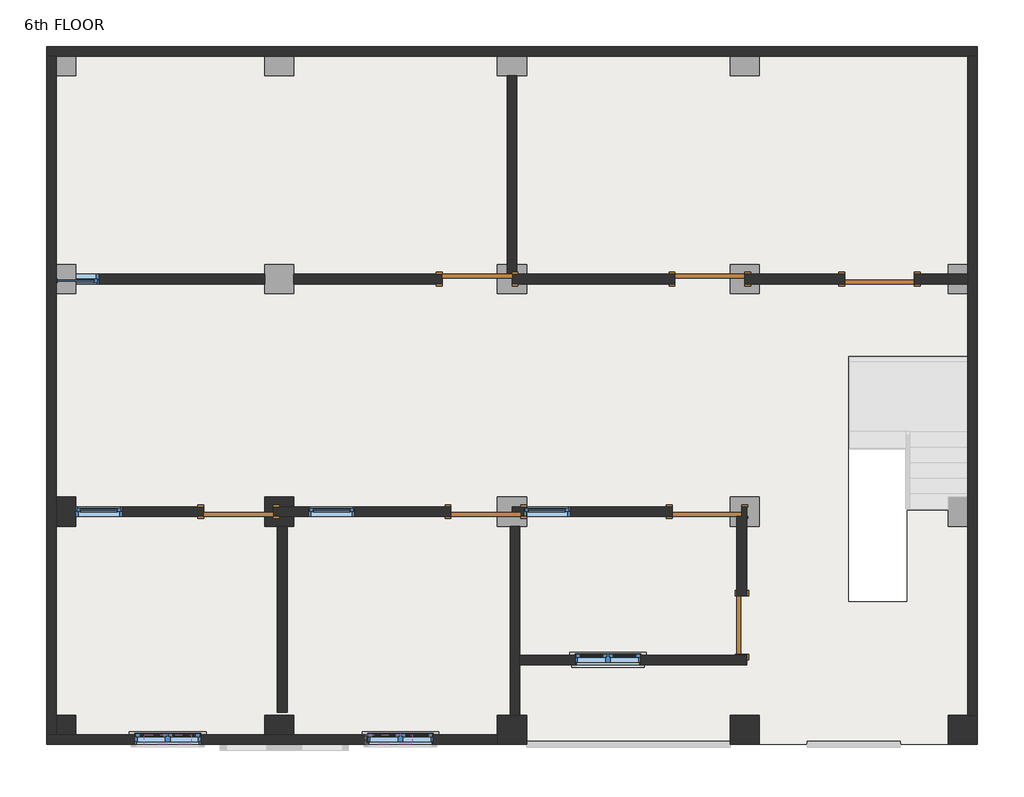
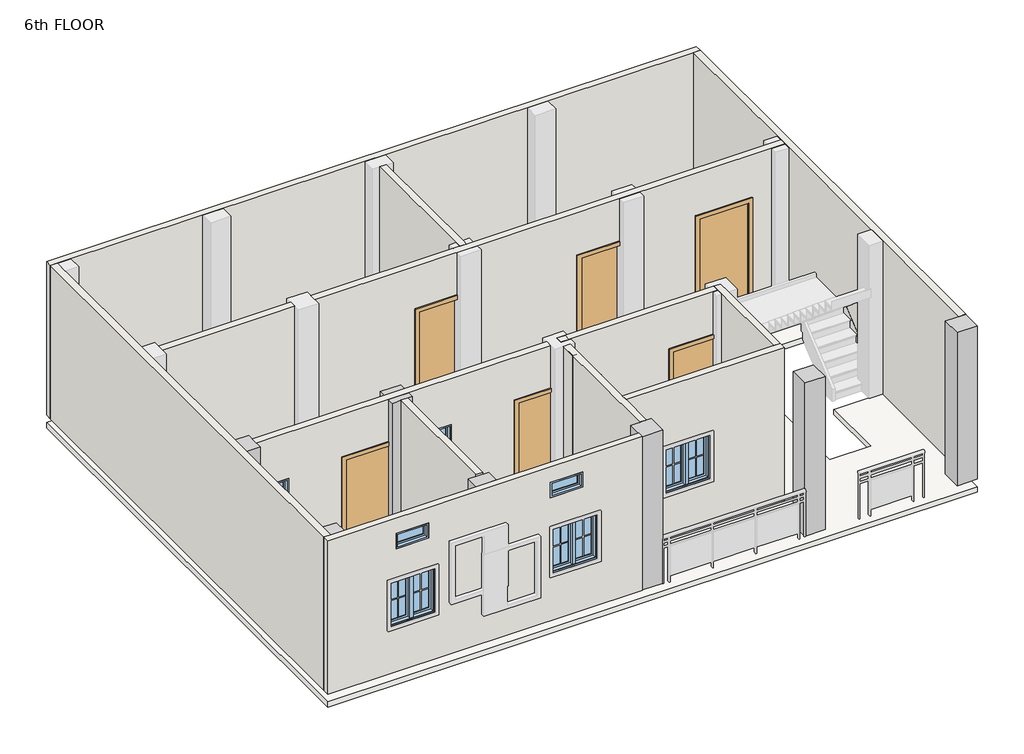
# One storey, part 1 of 2: 15 walls, 9 windows, 7 columns, 7 doors, 1 slab.
"""IFC4 building model written with IfcOpenShell, lengths in millimetres."""

from ifc_helpers import new_model, si_unit, frame, origin, place, context, project, spatial, polyline, outline, extrude, faceted_brep, transform, mapped, element, save
from components import door_e00f436c, door_a1797ceb, window_4c2727af, window_0bf3737e, window_78893e6c, window_0d9958e7

model = new_model("IFC4")

# Units and contexts
model_context = context("Model", 3, world=origin())
ifc_project = project(units=[si_unit("LENGTHUNIT", "METRE", prefix="MILLI")], contexts=[model_context])

# Site, building, storey
site = spatial("IfcSite", under=ifc_project)
building = spatial("IfcBuilding", under=site)
storey = spatial("IfcBuildingStorey", under=building, Name="6th FLOOR", Elevation=18135.6)

# Columns
placement = place(None, origin())
element("IfcColumn", 1, ObjectType="column family : column family", at=placement, inside=storey, context=model_context, shape_type="Brep", body=[
    faceted_brep([(-12576.097125, 2486.2065522, 18140.6), (-12957.097125, 2486.2065522, 18140.6), (-12957.097125, 2867.2065522, 18140.6), (-12576.097125, 2867.2065522, 18140.6), (-12576.097125, 2740.2065522, 18140.6), (-12842.797125, 2740.2065522, 18140.6), (-12842.797125, 2613.2065522, 18140.6), (-12576.097125, 2613.2065522, 18140.6), (-12576.097125, 2486.2065522, 21178.6), (-12576.097125, 2613.2065522, 21178.6), (-12957.097125, 2486.2065522, 21178.6), (-12957.097125, 2613.2065522, 21178.6), (-12957.097125, 2613.2065522, 20269.2), (-12957.097125, 2740.2065522, 20269.2), (-12957.097125, 2740.2065522, 21178.6), (-12957.097125, 2867.2065522, 21178.6), (-12576.097125, 2867.2065522, 21178.6), (-12842.797125, 2613.2065522, 20269.2), (-12842.797125, 2740.2065522, 20269.2), (-12576.097125, 2740.2065522, 21178.6)], [[[0, 1, 2, 3, 4, 5, 6, 7]], [[8, 0, 7, 9]], [[1, 0, 8, 10]], [[2, 1, 10, 11, 12, 13, 14, 15]], [[3, 2, 15, 16]], [[10, 8, 9, 11]], [[6, 17, 12, 11, 9, 7]], [[13, 18, 5, 4, 19, 14]], [[3, 16, 19, 4]], [[16, 15, 14, 19]], [[17, 18, 13, 12]], [[18, 17, 6, 5]]]),
])
element("IfcColumn", 2, ObjectType="column family : column family", at=placement, inside=storey, context=model_context, shape_type="SweptSolid", body=[
    extrude(outline(polyline([(-15433.597125, 2867.2065522), (-15433.597125, 2486.2065522), (-15687.597125, 2486.2065522), (-15687.597125, 2867.2065522), (-15433.597125, 2867.2065522)])), frame((0.0, 0.0, 18140.6), z_axis=(0.0, 0.0, 1.0), x_axis=(1.0, 0.0, 0.0)), (0.0, 0.0, 1.0), 3038.0),
])
element("IfcColumn", 3, ObjectType="column family : column family", at=placement, inside=storey, context=model_context, shape_type="SweptSolid", body=[
    extrude(outline(polyline([(-15433.597125, 9.7065522), (-15433.597125, -244.2934478), (-15687.597125, -244.2934478), (-15687.597125, 9.7065522), (-15433.597125, 9.7065522)])), frame((0.0, 0.0, 18140.6), z_axis=(0.0, 0.0, 1.0), x_axis=(1.0, 0.0, 0.0)), (0.0, 0.0, 1.0), 3038.0),
])
element("IfcColumn", 4, ObjectType="column family : column family", at=placement, inside=storey, context=model_context, shape_type="SweptSolid", body=[
    extrude(outline(polyline([(-3622.597125, 9.7065522), (-3622.597125, -371.2934478), (-4003.597125, -371.2934478), (-4003.597125, 9.7065522), (-3622.597125, 9.7065522)])), frame((0.0, 0.0, 18140.6), z_axis=(0.0, 0.0, 1.0), x_axis=(1.0, 0.0, 0.0)), (0.0, 0.0, 1.0), 3038.0),
])
element("IfcColumn", 5, ObjectType="column family : column family", at=placement, inside=storey, context=model_context, shape_type="SweptSolid", body=[
    extrude(outline(polyline([(-6480.097125, 9.7065522), (-6480.097125, -371.2934478), (-6861.097125, -371.2934478), (-6861.097125, 9.7065522), (-6480.097125, 9.7065522)])), frame((0.0, 0.0, 18140.6), z_axis=(0.0, 0.0, 1.0), x_axis=(1.0, 0.0, 0.0)), (0.0, 0.0, 1.0), 3038.0),
])
element("IfcColumn", 6, ObjectType="column family : column family", at=placement, inside=storey, context=model_context, shape_type="SweptSolid", body=[
    extrude(outline(polyline([(-9528.097125, 9.7065522), (-9528.097125, -371.2934478), (-9909.097125, -371.2934478), (-9909.097125, 9.7065522), (-9528.097125, 9.7065522)])), frame((0.0, 0.0, 18140.6), z_axis=(0.0, 0.0, 1.0), x_axis=(1.0, 0.0, 0.0)), (0.0, 0.0, 1.0), 3038.0),
])
element("IfcColumn", 7, ObjectType="column family : column family", at=placement, inside=storey, context=model_context, shape_type="SweptSolid", body=[
    extrude(outline(polyline([(-12957.097125, 9.7065522), (-12576.097125, 9.7065522), (-12576.097125, -244.2934478), (-12957.097125, -244.2934478), (-12957.097125, 9.7065522)])), frame((0.0, 0.0, 18140.6), z_axis=(0.0, 0.0, 1.0), x_axis=(1.0, 0.0, 0.0)), (0.0, 0.0, 1.0), 3038.0),
])

# Doors
door_shape = door_e00f436c(model_context)
element("IfcDoor", 8, ObjectType="Single-Flush : 30\" x 80\"", at=placement, inside=storey, context=model_context, shape_type="MappedRepresentation", body=[
    mapped(door_shape, transform((-6708.697125, 1190.8065522, 18135.6), x_axis=(0.0, -1.0, 0.0), y_axis=(1.0, 0.0, 0.0), z_axis=(0.0, 0.0, 1.0))),
])
door_2_shape = door_a1797ceb(model_context)
element("IfcDoor", 9, ObjectType="Single-Flush : 36\" x 84\"", at=placement, inside=storey, context=model_context, shape_type="MappedRepresentation", body=[
    mapped(door_2_shape, transform((-10175.797125, 5724.7065522, 18135.6), x_axis=(1.0, 0.0, 0.0), y_axis=(0.0, 1.0, 0.0), z_axis=(0.0, 0.0, 1.0))),
])
element("IfcDoor", 10, ObjectType="Single-Flush : 36\" x 84\"", at=placement, inside=storey, context=model_context, shape_type="MappedRepresentation", body=[
    mapped(door_2_shape, transform((-10061.497125, 2676.7065522, 18135.6), x_axis=(-1.0, 0.0, 0.0), y_axis=(0.0, -1.0, 0.0), z_axis=(0.0, 0.0, 1.0))),
])
element("IfcDoor", 11, ObjectType="Single-Flush : 36\" x 84\"", at=placement, inside=storey, context=model_context, shape_type="MappedRepresentation", body=[
    mapped(door_2_shape, transform((-13299.997125, 2676.7065522, 18135.6), x_axis=(-1.0, 0.0, 0.0), y_axis=(0.0, -1.0, 0.0), z_axis=(0.0, 0.0, 1.0))),
])
element("IfcDoor", 12, ObjectType="Single-Flush : 36\" x 84\"", at=placement, inside=storey, context=model_context, shape_type="MappedRepresentation", body=[
    mapped(door_2_shape, transform((-7127.797125, 5724.7065522, 18135.6), x_axis=(1.0, 0.0, 0.0), y_axis=(0.0, 1.0, 0.0), z_axis=(0.0, 0.0, 1.0))),
])
element("IfcDoor", 13, ObjectType="Single-Flush : 36\" x 84\"", at=placement, inside=storey, context=model_context, shape_type="MappedRepresentation", body=[
    mapped(door_2_shape, transform((-7165.897125, 2676.7065522, 18135.6), x_axis=(-1.0, 0.0, 0.0), y_axis=(0.0, -1.0, 0.0), z_axis=(0.0, 0.0, 1.0))),
])
element("IfcDoor", 14, ObjectType="Single-Flush : 36\" x 84\"", at=placement, inside=storey, context=model_context, shape_type="MappedRepresentation", body=[
    mapped(door_2_shape, transform((-4905.297125, 5724.7065522, 18135.6), x_axis=(-1.0, 0.0, 0.0), y_axis=(0.0, -1.0, 0.0), z_axis=(0.0, 0.0, 1.0))),
])

# Slab
element("IfcSlab", 15, ObjectType="Generic - 4\"", at=placement, inside=storey, context=model_context, shape_type="SweptSolid", body=[
    extrude(outline(polyline([(-3622.597125, 8772.7065522), (-3622.597125, -371.2934478), (-15814.597125, -371.2934478), (-15814.597125, 8772.7065522), (-3622.597125, 8772.7065522)]), holes=[polyline([(-3734.357125, 4711.0719226), (-5310.2646464, 4711.0719226), (-5310.2646464, 1502.3126957), (-4547.7736682, 1502.3126957), (-4547.7736682, 2699.911213), (-3734.357125, 2699.911213), (-3734.357125, 4711.0719226)])]), frame((0.0, 0.0, 17881.6), z_axis=(0.0, 0.0, 1.0), x_axis=(1.0, 0.0, 0.0)), (0.0, 0.0, 1.0), 101.6),
])

# Walls
element("IfcWall", 16, ObjectType="Generic - 5\"", at=placement, inside=storey, context=model_context, shape_type="Brep", body=[
    faceted_brep([(-15814.597125, 8645.7065522, 18135.6), (-15687.597125, 8645.7065522, 18135.6), (-3749.597125, 8645.7065522, 18135.6), (-3622.597125, 8645.7065522, 18135.6), (-3622.597125, 8645.7065522, 21183.6), (-3749.597125, 8645.7065522, 21183.6), (-15687.597125, 8645.7065522, 21183.6), (-15814.597125, 8645.7065522, 21183.6), (-15814.597125, 8772.7065522, 18135.6), (-15814.597125, 8772.7065522, 21183.6), (-3622.597125, 8772.7065522, 21183.6), (-3622.597125, 8772.7065522, 18135.6)], [[[0, 1, 2, 3, 4, 5, 6, 7]], [[8, 9, 10, 11]], [[3, 2, 1, 0, 8, 11]], [[7, 6, 5, 4, 10, 9]], [[4, 3, 11, 10]], [[0, 7, 9, 8]]]),
])
element("IfcWall", 17, ObjectType="Generic - 5\"", at=placement, inside=storey, context=model_context, shape_type="Brep", body=[
    faceted_brep([(-3749.597125, 8645.7065522, 18135.6), (-3749.597125, 5788.2065522, 18135.6), (-3749.597125, 5661.2065522, 18135.6), (-3749.597125, 9.7065522, 18135.6), (-3749.597125, 9.7065522, 21183.6), (-3749.597125, 5661.2065522, 21183.6), (-3749.597125, 5788.2065522, 21183.6), (-3749.597125, 8645.7065522, 21183.6), (-3622.597125, 8645.7065522, 18135.6), (-3622.597125, 8645.7065522, 21183.6), (-3622.597125, 9.7065522, 21183.6), (-3622.597125, 9.7065522, 21178.6), (-3622.597125, 9.7065522, 18140.6), (-3622.597125, 9.7065522, 18135.6)], [[[0, 1, 2, 3, 4, 5, 6, 7]], [[8, 9, 10, 11, 12, 13]], [[3, 2, 1, 0, 8, 13]], [[4, 3, 13, 12, 11, 10]], [[7, 6, 5, 4, 10, 9]], [[0, 7, 9, 8]]]),
])
element("IfcWall", 18, ObjectType="Generic - 5\"", at=placement, inside=storey, context=model_context, shape_type="Brep", body=[
    faceted_brep([(-9909.097125, -244.2934478, 18135.6), (-15687.597125, -244.2934478, 18135.6), (-15814.597125, -244.2934478, 18135.6), (-15814.597125, -244.2934478, 21183.6), (-15687.597125, -244.2934478, 21183.6), (-9909.097125, -244.2934478, 21183.6), (-13795.297125, -244.2934478, 19964.4), (-14658.897125, -244.2934478, 19964.4), (-14658.897125, -244.2934478, 19050.0), (-13795.297125, -244.2934478, 19050.0), (-10747.297125, -244.2934478, 19964.4), (-11610.897125, -244.2934478, 19964.4), (-11610.897125, -244.2934478, 19050.0), (-10747.297125, -244.2934478, 19050.0), (-13922.297125, -244.2934478, 20878.8), (-14531.897125, -244.2934478, 20878.8), (-14531.897125, -244.2934478, 20574.0), (-13922.297125, -244.2934478, 20574.0), (-11026.697125, -244.2934478, 20878.8), (-11636.297125, -244.2934478, 20878.8), (-11636.297125, -244.2934478, 20574.0), (-11026.697125, -244.2934478, 20574.0), (-9909.097125, -371.2934478, 18135.6), (-9909.097125, -371.2934478, 18140.6), (-9909.097125, -371.2934478, 21178.6), (-9909.097125, -371.2934478, 21183.6), (-15814.597125, -371.2934478, 21183.6), (-15814.597125, -371.2934478, 18135.6), (-13795.297125, -371.2934478, 19964.4), (-13795.297125, -371.2934478, 19050.0), (-14658.897125, -371.2934478, 19050.0), (-14658.897125, -371.2934478, 19964.4), (-10747.297125, -371.2934478, 19964.4), (-10747.297125, -371.2934478, 19050.0), (-11610.897125, -371.2934478, 19050.0), (-11610.897125, -371.2934478, 19964.4), (-13922.297125, -371.2934478, 20878.8), (-13922.297125, -371.2934478, 20574.0), (-14531.897125, -371.2934478, 20574.0), (-14531.897125, -371.2934478, 20878.8), (-11026.697125, -371.2934478, 20878.8), (-11026.697125, -371.2934478, 20574.0), (-11636.297125, -371.2934478, 20574.0), (-11636.297125, -371.2934478, 20878.8)], [[[0, 1, 2, 3, 4, 5], [6, 7, 8, 9], [10, 11, 12, 13], [14, 15, 16, 17], [18, 19, 20, 21]], [[22, 23, 24, 25, 26, 27], [28, 29, 30, 31], [32, 33, 34, 35], [36, 37, 38, 39], [40, 41, 42, 43]], [[2, 1, 0, 22, 27]], [[5, 4, 3, 26, 25]], [[0, 5, 25, 24, 23, 22]], [[3, 2, 27, 26]], [[29, 28, 6, 9]], [[30, 29, 9, 8]], [[31, 30, 8, 7]], [[28, 31, 7, 6]], [[33, 32, 10, 13]], [[34, 33, 13, 12]], [[35, 34, 12, 11]], [[32, 35, 11, 10]], [[37, 36, 14, 17]], [[38, 37, 17, 16]], [[39, 38, 16, 15]], [[36, 39, 15, 14]], [[41, 40, 18, 21]], [[42, 41, 21, 20]], [[43, 42, 20, 19]], [[40, 43, 19, 18]]]),
])
element("IfcWall", 19, ObjectType="Generic - 5\"", at=placement, inside=storey, context=model_context, shape_type="Brep", body=[
    faceted_brep([(-15687.597125, -244.2934478, 18135.6), (-15687.597125, 8645.7065522, 18135.6), (-15687.597125, 8645.7065522, 18140.6), (-15687.597125, 8645.7065522, 21178.6), (-15687.597125, 8645.7065522, 21183.6), (-15687.597125, -244.2934478, 21183.6), (-15687.597125, -244.2934478, 21178.6), (-15687.597125, -244.2934478, 18140.6), (-15814.597125, -244.2934478, 18135.6), (-15814.597125, -244.2934478, 21183.6), (-15814.597125, 8645.7065522, 21183.6), (-15814.597125, 8645.7065522, 18135.6)], [[[0, 1, 2, 3, 4, 5, 6, 7]], [[8, 9, 10, 11]], [[1, 0, 8, 11]], [[5, 4, 10, 9]], [[4, 3, 2, 1, 11, 10]], [[0, 7, 6, 5, 9, 8]]]),
])
element("IfcWall", 20, ObjectType="Generic - 5\"", at=placement, inside=storey, context=model_context, shape_type="SweptSolid", body=[
    extrude(outline(polyline([(18135.6, -15433.597125), (18135.6, -12957.097125), (21183.6, -12957.097125), (21183.6, -15433.597125), (20269.2, -15433.597125), (20269.2, -15128.797125), (18440.4, -15128.797125), (18440.4, -15433.597125), (18135.6, -15433.597125)])), frame((0.0, 5661.2065522, 0.0), z_axis=(0.0, 1.0, 0.0), x_axis=(0.0, 0.0, 1.0)), (0.0, 0.0, 1.0), 127.0),
])
element("IfcWall", 21, ObjectType="Generic - 5\"", at=placement, inside=storey, context=model_context, shape_type="Brep", body=[
    faceted_brep([(-9782.097125, 8391.7065522, 18135.6), (-9782.097125, 5788.2065522, 18135.6), (-9782.097125, 5788.2065522, 18140.6), (-9782.097125, 5788.2065522, 20269.2), (-9782.097125, 5788.2065522, 21178.6), (-9782.097125, 5788.2065522, 21183.6), (-9782.097125, 8391.7065522, 21183.6), (-9655.097125, 8391.7065522, 18135.6), (-9655.097125, 8391.7065522, 21183.6), (-9655.097125, 5788.2065522, 21183.6), (-9655.097125, 5788.2065522, 21178.6), (-9655.097125, 5788.2065522, 18140.6), (-9655.097125, 5788.2065522, 18135.6), (-9718.597125, 5788.2065522, 18135.6)], [[[0, 1, 2, 3, 4, 5, 6]], [[7, 8, 9, 10, 11, 12]], [[1, 0, 7, 12, 13]], [[6, 5, 9, 8]], [[0, 6, 8, 7]], [[5, 4, 3, 2, 1, 13, 12, 11, 10, 9]]]),
])
element("IfcWall", 22, ObjectType="Generic - 5\"", at=placement, inside=storey, context=model_context, shape_type="Brep", body=[
    faceted_brep([(-6670.597125, 5661.2065522, 18135.6), (-5362.497125, 5661.2065522, 18135.6), (-5362.497125, 5661.2065522, 20269.2), (-4448.097125, 5661.2065522, 20269.2), (-4448.097125, 5661.2065522, 18135.6), (-3749.597125, 5661.2065522, 18135.6), (-3749.597125, 5661.2065522, 18140.6), (-3749.597125, 5661.2065522, 21178.6), (-3749.597125, 5661.2065522, 21183.6), (-12576.097125, 5661.2065522, 21183.6), (-12576.097125, 5661.2065522, 18135.6), (-10632.997125, 5661.2065522, 18135.6), (-10632.997125, 5661.2065522, 20269.2), (-9909.097125, 5661.2065522, 20269.2), (-9718.597125, 5661.2065522, 20269.2), (-9718.597125, 5661.2065522, 18140.6), (-9718.597125, 5661.2065522, 18135.6), (-7584.997125, 5661.2065522, 18135.6), (-7584.997125, 5661.2065522, 20269.2), (-6861.097125, 5661.2065522, 20269.2), (-6670.597125, 5661.2065522, 20269.2), (-6670.597125, 5661.2065522, 18140.6), (-5362.497125, 5788.2065522, 20269.2), (-5362.497125, 5788.2065522, 18135.6), (-6670.597125, 5788.2065522, 18135.6), (-6670.597125, 5788.2065522, 18140.6), (-6670.597125, 5788.2065522, 20269.2), (-6861.097125, 5788.2065522, 20269.2), (-7584.997125, 5788.2065522, 20269.2), (-7584.997125, 5788.2065522, 18135.6), (-9655.097125, 5788.2065522, 18135.6), (-9718.597125, 5788.2065522, 18135.6), (-9718.597125, 5788.2065522, 18140.6), (-9718.597125, 5788.2065522, 20269.2), (-9782.097125, 5788.2065522, 20269.2), (-9909.097125, 5788.2065522, 20269.2), (-10632.997125, 5788.2065522, 20269.2), (-10632.997125, 5788.2065522, 18135.6), (-12576.097125, 5788.2065522, 18135.6), (-12576.097125, 5788.2065522, 21183.6), (-9782.097125, 5788.2065522, 21183.6), (-9655.097125, 5788.2065522, 21183.6), (-3749.597125, 5788.2065522, 21183.6), (-3749.597125, 5788.2065522, 21178.6), (-3749.597125, 5788.2065522, 18140.6), (-3749.597125, 5788.2065522, 18135.6), (-4448.097125, 5788.2065522, 18135.6), (-4448.097125, 5788.2065522, 20269.2)], [[[0, 1, 2, 3, 4, 5, 6, 7, 8, 9, 10, 11, 12, 13, 14, 15, 16, 17, 18, 19, 20, 21]], [[22, 23, 24, 25, 26, 27, 28, 29, 30, 31, 32, 33, 34, 35, 36, 37, 38, 39, 40, 41, 42, 43, 44, 45, 46, 47]], [[11, 10, 38, 37]], [[17, 16, 31, 30, 29]], [[46, 45, 5, 4]], [[24, 23, 1, 0]], [[9, 8, 42, 41, 40, 39]], [[10, 9, 39, 38]], [[8, 7, 6, 5, 45, 44, 43, 42]], [[33, 32, 31, 16, 15, 14]], [[36, 35, 34, 33, 14, 13, 12]], [[37, 36, 12, 11]], [[26, 25, 24, 0, 21, 20]], [[28, 27, 26, 20, 19, 18]], [[29, 28, 18, 17]], [[2, 1, 23, 22]], [[3, 2, 22, 47]], [[4, 3, 47, 46]]]),
])
element("IfcWall", 23, ObjectType="Generic - 5\"", at=placement, inside=storey, context=model_context, shape_type="Brep", body=[
    faceted_brep([(-14823.997125, 2613.2065522, 18440.4), (-15433.597125, 2613.2065522, 18440.4), (-15433.597125, 2613.2065522, 18135.6), (-13757.197125, 2613.2065522, 18135.6), (-13757.197125, 2613.2065522, 20269.2), (-12957.097125, 2613.2065522, 20269.2), (-12842.797125, 2613.2065522, 20269.2), (-12842.797125, 2613.2065522, 18140.6), (-12842.797125, 2613.2065522, 18135.6), (-10518.697125, 2613.2065522, 18135.6), (-10518.697125, 2613.2065522, 20269.2), (-9909.097125, 2613.2065522, 20269.2), (-9909.097125, 2613.2065522, 21183.6), (-15433.597125, 2613.2065522, 21183.6), (-15433.597125, 2613.2065522, 20269.2), (-14823.997125, 2613.2065522, 20269.2), (-12385.597125, 2613.2065522, 20269.2), (-11775.997125, 2613.2065522, 20269.2), (-11775.997125, 2613.2065522, 18440.4), (-12385.597125, 2613.2065522, 18440.4), (-15433.597125, 2740.2065522, 18135.6), (-15433.597125, 2740.2065522, 18440.4), (-14823.997125, 2740.2065522, 18440.4), (-14823.997125, 2740.2065522, 20269.2), (-15433.597125, 2740.2065522, 20269.2), (-15433.597125, 2740.2065522, 21183.6), (-9909.097125, 2740.2065522, 21183.6), (-9909.097125, 2740.2065522, 20269.2), (-10518.697125, 2740.2065522, 20269.2), (-10518.697125, 2740.2065522, 18135.6), (-12842.797125, 2740.2065522, 18135.6), (-12842.797125, 2740.2065522, 18140.6), (-12842.797125, 2740.2065522, 20269.2), (-12957.097125, 2740.2065522, 20269.2), (-13757.197125, 2740.2065522, 20269.2), (-13757.197125, 2740.2065522, 18135.6), (-12385.597125, 2740.2065522, 20269.2), (-12385.597125, 2740.2065522, 18440.4), (-11775.997125, 2740.2065522, 18440.4), (-11775.997125, 2740.2065522, 20269.2)], [[[0, 1, 2, 3, 4, 5, 6, 7, 8, 9, 10, 11, 12, 13, 14, 15], [16, 17, 18, 19]], [[20, 21, 22, 23, 24, 25, 26, 27, 28, 29, 30, 31, 32, 33, 34, 35], [36, 37, 38, 39]], [[30, 29, 9, 8]], [[20, 35, 3, 2]], [[26, 12, 11, 27]], [[13, 12, 26, 25]], [[14, 13, 25, 24]], [[2, 1, 21, 20]], [[28, 10, 9, 29]], [[10, 28, 27, 11]], [[4, 3, 35, 34]], [[6, 5, 4, 34, 33, 32]], [[8, 7, 6, 32, 31, 30]], [[22, 21, 1, 0]], [[23, 22, 0, 15]], [[24, 23, 15, 14]], [[37, 36, 16, 19]], [[38, 37, 19, 18]], [[39, 38, 18, 17]], [[36, 39, 17, 16]]]),
])
element("IfcWall", 24, ObjectType="Generic - 5\"", at=placement, inside=storey, context=model_context, shape_type="Brep", body=[
    faceted_brep([(-9616.997125, 9.7065522, 18135.6), (-9616.997125, 670.1065522, 18135.6), (-9616.997125, 797.1065522, 18135.6), (-9616.997125, 2486.2065522, 18135.6), (-9616.997125, 2486.2065522, 21183.6), (-9616.997125, 797.1065522, 21183.6), (-9616.997125, 670.1065522, 21183.6), (-9616.997125, 9.7065522, 21183.6), (-9743.997125, 9.7065522, 18135.6), (-9743.997125, 9.7065522, 21183.6), (-9743.997125, 2486.2065522, 21183.6), (-9743.997125, 2486.2065522, 18135.6)], [[[0, 1, 2, 3, 4, 5, 6, 7]], [[8, 9, 10, 11]], [[3, 2, 1, 0, 8, 11]], [[4, 3, 11, 10]], [[7, 6, 5, 4, 10, 9]], [[0, 7, 9, 8]]]),
])
element("IfcWall", 25, ObjectType="Generic - 5\"", at=placement, inside=storey, context=model_context, shape_type="SweptSolid", body=[
    extrude(outline(polyline([(-9743.997125, 2181.4065522), (-9743.997125, 2486.2065522), (-9616.997125, 2486.2065522), (-9616.997125, 2181.4065522), (-9743.997125, 2181.4065522)])), frame((0.0, 0.0, 18135.6), z_axis=(0.0, 0.0, 1.0), x_axis=(1.0, 0.0, 0.0)), (0.0, 0.0, 1.0), 3048.0),
])
element("IfcWall", 26, ObjectType="Generic - 5\"", at=placement, inside=storey, context=model_context, shape_type="Brep", body=[
    faceted_brep([(-6772.197125, 2613.2065522, 21183.6), (-9718.597125, 2613.2065522, 21183.6), (-9718.597125, 2613.2065522, 21178.6), (-9718.597125, 2613.2065522, 18140.6), (-9718.597125, 2613.2065522, 18135.6), (-7623.097125, 2613.2065522, 18135.6), (-7623.097125, 2613.2065522, 20269.2), (-6861.097125, 2613.2065522, 20269.2), (-6772.197125, 2613.2065522, 20269.2), (-6772.197125, 2613.2065522, 21178.6), (-9566.197125, 2613.2065522, 20269.2), (-9528.097125, 2613.2065522, 20269.2), (-8956.597125, 2613.2065522, 20269.2), (-8956.597125, 2613.2065522, 18440.4), (-9528.097125, 2613.2065522, 18440.4), (-9566.197125, 2613.2065522, 18440.4), (-9718.597125, 2740.2065522, 21183.6), (-6772.197125, 2740.2065522, 21183.6), (-6772.197125, 2740.2065522, 20269.2), (-6861.097125, 2740.2065522, 20269.2), (-7623.097125, 2740.2065522, 20269.2), (-7623.097125, 2740.2065522, 18135.6), (-9718.597125, 2740.2065522, 18135.6), (-9718.597125, 2740.2065522, 18140.6), (-9718.597125, 2740.2065522, 21178.6), (-9566.197125, 2740.2065522, 20269.2), (-9566.197125, 2740.2065522, 18440.4), (-9528.097125, 2740.2065522, 18440.4), (-8956.597125, 2740.2065522, 18440.4), (-8956.597125, 2740.2065522, 20269.2), (-9528.097125, 2740.2065522, 20269.2)], [[[0, 1, 2, 3, 4, 5, 6, 7, 8, 9], [10, 11, 12, 13, 14, 15]], [[16, 17, 18, 19, 20, 21, 22, 23, 24], [25, 26, 27, 28, 29, 30]], [[4, 22, 21, 5]], [[1, 0, 17, 16]], [[4, 3, 2, 1, 16, 24, 23, 22]], [[26, 25, 10, 15]], [[28, 27, 26, 15, 14, 13]], [[29, 28, 13, 12]], [[25, 30, 29, 12, 11, 10]], [[20, 6, 5, 21]], [[6, 20, 19, 18, 8, 7]], [[17, 0, 9, 8, 18]]]),
])
element("IfcWall", 27, ObjectType="Generic - 5\"", at=placement, inside=storey, context=model_context, shape_type="Brep", body=[
    faceted_brep([(-6645.197125, 797.1065522, 18135.6), (-6645.197125, 809.8065522, 18135.6), (-6645.197125, 809.8065522, 20167.6), (-6645.197125, 1571.8065522, 20167.6), (-6645.197125, 1571.8065522, 18135.6), (-6645.197125, 2740.2065522, 18135.6), (-6645.197125, 2740.2065522, 18140.6), (-6645.197125, 2740.2065522, 21178.6), (-6645.197125, 2740.2065522, 21183.6), (-6645.197125, 797.1065522, 21183.6), (-6772.197125, 809.8065522, 20167.6), (-6772.197125, 809.8065522, 18135.6), (-6772.197125, 797.1065522, 18135.6), (-6772.197125, 797.1065522, 21183.6), (-6772.197125, 2613.2065522, 21183.6), (-6772.197125, 2740.2065522, 21183.6), (-6772.197125, 2740.2065522, 20269.2), (-6772.197125, 2613.2065522, 20269.2), (-6772.197125, 2613.2065522, 18140.6), (-6772.197125, 2613.2065522, 18135.6), (-6772.197125, 1571.8065522, 18135.6), (-6772.197125, 1571.8065522, 20167.6), (-6708.697125, 2613.2065522, 18135.6), (-6708.697125, 2740.2065522, 18135.6), (-6708.697125, 2613.2065522, 20269.2), (-6708.697125, 2613.2065522, 18140.6), (-6708.697125, 2740.2065522, 20269.2), (-6708.697125, 2740.2065522, 18140.6)], [[[0, 1, 2, 3, 4, 5, 6, 7, 8, 9]], [[10, 11, 12, 13, 14, 15, 16, 17, 18, 19, 20, 21]], [[20, 19, 22, 23, 5, 4]], [[12, 11, 1, 0]], [[9, 8, 15, 14, 13]], [[24, 25, 22, 19, 18, 17]], [[26, 24, 17, 16]], [[22, 25, 24, 26, 27, 23]], [[8, 7, 6, 5, 23, 27, 26, 16, 15]], [[0, 9, 13, 12]], [[2, 1, 11, 10]], [[3, 2, 10, 21]], [[4, 3, 21, 20]]]),
])
element("IfcWall", 28, ObjectType="Generic - 5\"", at=placement, inside=storey, context=model_context, shape_type="Brep", body=[
    faceted_brep([(-9718.597125, 2613.2065522, 18135.6), (-9566.197125, 2613.2065522, 18135.6), (-9566.197125, 2613.2065522, 18440.4), (-9566.197125, 2613.2065522, 20269.2), (-9566.197125, 2613.2065522, 21183.6), (-9718.597125, 2613.2065522, 21183.6), (-9718.597125, 2613.2065522, 21178.6), (-9718.597125, 2613.2065522, 18140.6), (-9718.597125, 2740.2065522, 18135.6), (-9718.597125, 2740.2065522, 18140.6), (-9718.597125, 2740.2065522, 21178.6), (-9718.597125, 2740.2065522, 21183.6), (-9566.197125, 2740.2065522, 21183.6), (-9566.197125, 2740.2065522, 20269.2), (-9566.197125, 2740.2065522, 18440.4), (-9566.197125, 2740.2065522, 18135.6)], [[[0, 1, 2, 3, 4, 5, 6, 7]], [[8, 9, 10, 11, 12, 13, 14, 15]], [[1, 0, 8, 15]], [[4, 3, 2, 1, 15, 14, 13, 12]], [[5, 4, 12, 11]], [[0, 7, 6, 5, 11, 10, 9, 8]]]),
])
element("IfcWall", 29, ObjectType="Generic - 5\"", at=placement, inside=storey, context=model_context, shape_type="SweptSolid", body=[
    extrude(outline(polyline([(-12791.997125, 47.8065522), (-12791.997125, 2486.2065522), (-12664.997125, 2486.2065522), (-12664.997125, 47.8065522), (-12791.997125, 47.8065522)])), frame((0.0, 0.0, 18135.6), z_axis=(0.0, 0.0, 1.0), x_axis=(1.0, 0.0, 0.0)), (0.0, 0.0, 1.0), 3048.0),
])
element("IfcWall", 30, ObjectType="Generic - 5\"", at=placement, inside=storey, context=model_context, shape_type="Brep", body=[
    faceted_brep([(-9616.997125, 670.1065522, 18135.6), (-6645.197125, 670.1065522, 18135.6), (-6645.197125, 670.1065522, 21183.6), (-9616.997125, 670.1065522, 21183.6), (-8029.497125, 670.1065522, 19964.4), (-8029.497125, 670.1065522, 19050.0), (-8893.097125, 670.1065522, 19050.0), (-8893.097125, 670.1065522, 19964.4), (-9616.997125, 797.1065522, 18135.6), (-9616.997125, 797.1065522, 21183.6), (-6772.197125, 797.1065522, 21183.6), (-6645.197125, 797.1065522, 21183.6), (-6645.197125, 797.1065522, 18135.6), (-6772.197125, 797.1065522, 18135.6), (-8029.497125, 797.1065522, 19964.4), (-8893.097125, 797.1065522, 19964.4), (-8893.097125, 797.1065522, 19050.0), (-8029.497125, 797.1065522, 19050.0)], [[[0, 1, 2, 3], [4, 5, 6, 7]], [[8, 9, 10, 11, 12, 13], [14, 15, 16, 17]], [[1, 0, 8, 13, 12]], [[3, 2, 11, 10, 9]], [[0, 3, 9, 8]], [[2, 1, 12, 11]], [[5, 4, 14, 17]], [[6, 5, 17, 16]], [[7, 6, 16, 15]], [[4, 7, 15, 14]]]),
])

# Windows
window_shape = window_4c2727af(model_context)
element("IfcWindow", 31, ObjectType="Fixed : 24\" x 12\"", at=placement, inside=storey, context=model_context, shape_type="MappedRepresentation", body=[
    mapped(window_shape, transform((-14188.997125, -307.7934478, 19659.6), x_axis=(1.0, 0.0, 0.0), y_axis=(0.0, 1.0, 0.0), z_axis=(0.0, 0.0, 1.0))),
])
element("IfcWindow", 32, ObjectType="Fixed : 24\" x 12\"", at=placement, inside=storey, context=model_context, shape_type="MappedRepresentation", body=[
    mapped(window_shape, transform((-11293.397125, -307.7934478, 19659.6), x_axis=(1.0, 0.0, 0.0), y_axis=(0.0, 1.0, 0.0), z_axis=(0.0, 0.0, 1.0))),
])
window_2_shape = window_0bf3737e(model_context)
element("IfcWindow", 33, ObjectType="Fixed : 24\" x 72\"", at=placement, inside=storey, context=model_context, shape_type="MappedRepresentation", body=[
    mapped(window_2_shape, transform((-15471.697125, 5724.7065522, 18135.6), x_axis=(-1.0, 0.0, 0.0), y_axis=(0.0, -1.0, 0.0), z_axis=(0.0, 0.0, 1.0))),
])
window_3_shape = window_78893e6c(model_context)
element("IfcWindow", 34, ObjectType="Fixed : 24\" x 72\"", at=placement, inside=storey, context=model_context, shape_type="MappedRepresentation", body=[
    mapped(window_3_shape, transform((-15166.897125, 2676.7065522, 18135.6), x_axis=(-1.0, 0.0, 0.0), y_axis=(0.0, -1.0, 0.0), z_axis=(0.0, 0.0, 1.0))),
])
element("IfcWindow", 35, ObjectType="Fixed : 24\" x 72\"", at=placement, inside=storey, context=model_context, shape_type="MappedRepresentation", body=[
    mapped(window_3_shape, transform((-12118.897125, 2676.7065522, 18135.6), x_axis=(-1.0, 0.0, 0.0), y_axis=(0.0, -1.0, 0.0), z_axis=(0.0, 0.0, 1.0))),
])
element("IfcWindow", 36, ObjectType="Fixed : 24\" x 72\"", at=placement, inside=storey, context=model_context, shape_type="MappedRepresentation", body=[
    mapped(window_3_shape, transform((-9299.497125, 2676.7065522, 18135.6), x_axis=(-1.0, 0.0, 0.0), y_axis=(0.0, -1.0, 0.0), z_axis=(0.0, 0.0, 1.0))),
])
window_4_shape = window_0d9958e7(model_context)
element("IfcWindow", 37, ObjectType="Window-Casement-Double : 34\" x 36\"", at=placement, inside=storey, context=model_context, shape_type="MappedRepresentation", body=[
    mapped(window_4_shape, transform((-14227.097125, -307.7934478, 18135.6), x_axis=(1.0, 0.0, 0.0), y_axis=(0.0, 1.0, 0.0), z_axis=(0.0, 0.0, 1.0))),
])
element("IfcWindow", 38, ObjectType="Window-Casement-Double : 34\" x 36\"", at=placement, inside=storey, context=model_context, shape_type="MappedRepresentation", body=[
    mapped(window_4_shape, transform((-11179.097125, -307.7934478, 18135.6), x_axis=(1.0, 0.0, 0.0), y_axis=(0.0, 1.0, 0.0), z_axis=(0.0, 0.0, 1.0))),
])
element("IfcWindow", 39, ObjectType="Window-Casement-Double : 34\" x 36\"", at=placement, inside=storey, context=model_context, shape_type="MappedRepresentation", body=[
    mapped(window_4_shape, transform((-8461.297125, 733.6065522, 18135.6), x_axis=(1.0, 0.0, 0.0), y_axis=(0.0, 1.0, 0.0), z_axis=(0.0, 0.0, 1.0))),
])

save(model, "model.ifc")

# Revit data of these elements
# Type "column family : column family"
#   w2 [instance default] = 0' - 9.88189"
#   w1 [instance default] = 0' - 9.01575"
#   Depth = 1' - 11.62205"
#   Width = 1' - 11.62205"
# Type "Single-Flush : 30\" x 80\""
#   Type Mark = "5"
#   Construction Type Id = "MDOOR"
#   Assembly Code = "C1020"
#   Analytic Construction = "Metal"
#   Thickness = 0' - 2"
#   Heat Transfer Coefficient (U) = 0.651978 BTU/(h·ft²·°F)
#   Height = 6' - 8"
#   Trim Projection Ext = 0' - 1"
#   Trim Projection Int = 0' - 1"
#   Trim Width = 0' - 3"
#   Width = 2' - 6"
#   Define Thermal Properties by = 1
#   Define Thermal Properties by = 1
#   Door Material = Door - Panel
#   Frame Material = Door - Frame
#   Visual Light Transmittance = 0
#   Solar Heat Gain Coefficient = 0
#   Function = (empty or 0)
#   Wall Closure = (empty or 0)
# Type "Single-Flush : 36\" x 84\""
#   Type Mark = "1"
#   Construction Type Id = "MDOOR"
#   Assembly Code = "C1020"
#   Analytic Construction = "Metal"
#   Thickness = 0' - 2"
#   Heat Transfer Coefficient (U) = 0.651978 BTU/(h·ft²·°F)
#   Height = 7' - 0"
#   Trim Projection Ext = 0' - 1"
#   Trim Projection Int = 0' - 1"
#   Trim Width = 0' - 3"
#   Width = 3' - 0"
#   Define Thermal Properties by = 1
#   Define Thermal Properties by = 1
#   Door Material = Door - Panel
#   Frame Material = Door - Frame
#   Visual Light Transmittance = 0
#   Solar Heat Gain Coefficient = 0
#   Function = (empty or 0)
#   Wall Closure = (empty or 0)
# Type "Generic - 4\""
#   Assembly Code = "B1010"
#   Function = 0
#   Layers, outside or top first: 0' - 4" no material (function 1)
# Type "Generic - 5\""
#   Assembly Code = "B2010"
#   Layers, outside or top first: 0' - 5" no material (function 1)
# Type "Fixed : 24\" x 12\""
#   Type Mark = "4"
#   Construction Type Id = "GSP4R"
#   Assembly Code = "B2020100"
#   Analytic Construction = "1/8 in Pilkington single glazing"
#   Visual Light Transmittance = 0.9
#   Solar Heat Gain Coefficient = 0.78
#   Heat Transfer Coefficient (U) = 0.6496 BTU/(h·ft²·°F)
#   Height = 1' - 0"
#   Default Sill Height = 3' - 0"
#   Width = 2' - 0"
#   Window Inset = 0' - 0 3/4"
#   Define Thermal Properties by = 1
#   Define Thermal Properties by = 1
#   Glass Pane Material = Glass
#   Sash Material = Sash
#   Wall Closure = (empty or 0)
# Type "Fixed : 24\" x 72\""
#   Type Mark = "7"
#   Construction Type Id = "GSP4R"
#   Assembly Code = "B2020100"
#   Analytic Construction = "1/8 in Pilkington single glazing"
#   Visual Light Transmittance = 0.9
#   Solar Heat Gain Coefficient = 0.78
#   Heat Transfer Coefficient (U) = 0.6496 BTU/(h·ft²·°F)
#   Height = 6' - 0"
#   Default Sill Height = 1' - 0"
#   Width = 2' - 0"
#   Window Inset = 0' - 0 3/4"
#   Define Thermal Properties by = 1
#   Define Thermal Properties by = 1
#   Glass Pane Material = Glass
#   Sash Material = Sash
#   Wall Closure = (empty or 0)
# Type "Window-Casement-Double : 34\" x 36\""
#   Type Mark = "14"
#   Fire Rating = "0.5h"
#   Assembly Code = "B2020100"
#   Analytic Construction = "Double glazing - domestic"
#   Frame Extension [instance default] = 0' - 0 1/4"
#   Window Inset [instance default] = 0' - 0"
#   Wall Thickness [instance default] = 0' - 6"
#   Interior Wall Closure [instance default] = 0' - 2 1/4"
#   Half Width = 1' - 5"
#   Visual Light Transmittance = 0.81
#   Thermal Resistance (R) = 1.8146 (h·ft²·°F)/BTU
#   Solar Heat Gain Coefficient = 0.76
#   Rough Width = 2' - 10 1/2"
#   Rough Height = 3' - 0 1/2"
#   Height = 3' - 0"
#   Heat Transfer Coefficient (U) = 0.5511 BTU/(h·ft²·°F)
#   Exterior Wall Closure [instance default] = 0' - 1 1/4"
#   Extension Jamb [instance default] = 0' - 2 1/4"
#   Default Sill Height = 3' - 0"
#   Width = 2' - 10"
#   Define Thermal Properties by = 0
#   Muntin Visibility = yes
#   Interior Trim Visibility [instance default] = yes
#   Exterior Trim Visibility [instance default] = yes
#   Extension Jamb Visibility [instance default] = yes
#   Interior Trim Material = Wood - Stained
#   Muntin Pattern = Muntin Pattern_2x2 : Muntin Pattern_2x2
#   Interior Trim = Trim-Window-Interior-Flat : Picture Frame
#   Interior Frame Material = Wood - Stained
#   Glass Panel Material = Glass
#   Exterior Trim Material = Clad - White
#   Exterior Trim = Trim-Window-Exterior-Flat : with Sill
#   Exterior Frame Material = Clad - White
#   Wall Closure = (empty or 0)
# Element 1 (IfcColumn, "column family : column family")
#   w2 = 1' - 3"
#   w1 = 1' - 3"
#   Phase Created = New Construction
#   Materials on its faces: "Default Wall", "inside wall"
# Element 2 (IfcColumn, "column family : column family")
#   w2 = 1' - 3"
#   w1 = 0' - 10"
#   Phase Created = New Construction
#   Materials on its faces: "inside wall", "Default Wall"
# Elements 3, 7 (IfcColumn, "column family : column family")
#   w2 = 1' - 3"
#   w1 = 1' - 3"
#   Phase Created = New Construction
#   Materials on its faces: "Default Wall"
# Element 4 (IfcColumn, "column family : column family")
#   w2 = 1' - 3"
#   w1 = 1' - 3"
#   Phase Created = New Construction
#   Materials on its faces: "Clad - White", "Default Wall"
# Element 5 (IfcColumn, "column family : column family")
#   w2 = 1' - 3"
#   w1 = 1' - 3"
#   Phase Created = New Construction
#   Materials on its faces: "out side wall"
# Element 6 (IfcColumn, "column family : column family")
#   w2 = 1' - 3"
#   w1 = 1' - 3"
#   Phase Created = New Construction
#   Materials on its faces: "out side wall", "Default Wall"
# Element 8 (IfcDoor, "Single-Flush : 30\" x 80\"")
#   Phase Created = New Construction
#   Materials on its faces: "Door - Frame", "Door - Panel"
# Elements 9, 10, 11, 12, 13, 14 (IfcDoor, "Single-Flush : 36\" x 84\"")
#   Phase Created = New Construction
#   Materials on its faces: "Door - Frame", "Door - Panel"
# Element 15 (IfcSlab, "Generic - 4\"")
#   Height Offset From Level = -0' - 6"
#   Phase Created = New Construction
#   Materials on its faces: "Default Floor", "Clad - White", "floor"
# Element 16 (IfcWall, "Generic - 5\"")
#   Top Offset = 0' - 0"
#   Base Offset = 0' - 0"
#   wall height = 10' - 0"
#   Phase Created = New Construction
#   Base Constraint = 6th FLOOR
#   Top Constraint = 7th FLOOR
#   Materials on its faces: "Default Wall", "Clad - White"
# Element 17 (IfcWall, "Generic - 5\"")
#   Top Offset = 0' - 0"
#   Base Offset = 0' - 0"
#   wall height = 10' - 0"
#   Phase Created = New Construction
#   Base Constraint = 6th FLOOR
#   Top Constraint = 7th FLOOR
#   Materials on its faces: "Default Wall", "grey", "Clad - White"
# Element 18 (IfcWall, "Generic - 5\"")
#   Top Offset = 0' - 0"
#   Base Offset = 0' - 0"
#   wall height = 10' - 0"
#   Phase Created = New Construction
#   Base Constraint = 6th FLOOR
#   Top Constraint = 7th FLOOR
#   Materials on its faces: "Default Wall", "out side wall", "Clad - White"
# Element 19 (IfcWall, "Generic - 5\"")
#   Top Offset = 0' - 0"
#   Base Offset = 0' - 0"
#   wall height = 10' - 0"
#   Phase Created = New Construction
#   Base Constraint = 6th FLOOR
#   Top Constraint = 7th FLOOR
#   Materials on its faces: "Default Wall", "inside wall", "Clad - White"
# Elements 20, 23, 26, 27 (IfcWall, "Generic - 5\"")
#   Top Offset = 0' - 0"
#   Base Offset = 0' - 0"
#   wall height = 10' - 0"
#   Phase Created = New Construction
#   Base Constraint = 6th FLOOR
#   Top Constraint = 7th FLOOR
#   Materials on its faces: "Default Wall", "inside wall"
# Elements 21, 25, 28, 29 (IfcWall, "Generic - 5\"")
#   Top Offset = 0' - 0"
#   Base Offset = 0' - 0"
#   wall height = 10' - 0"
#   Phase Created = New Construction
#   Base Constraint = 6th FLOOR
#   Top Constraint = 7th FLOOR
#   Materials on its faces: "Default Wall"
# Elements 22, 24 (IfcWall, "Generic - 5\"")
#   Top Offset = 0' - 0"
#   Base Offset = 0' - 0"
#   wall height = 10' - 0"
#   Phase Created = New Construction
#   Base Constraint = 6th FLOOR
#   Top Constraint = 7th FLOOR
#   Materials on its faces: "Default Wall", "grey"
# Element 30 (IfcWall, "Generic - 5\"")
#   Top Offset = 0' - 0"
#   Base Offset = 0' - 0"
#   wall height = 10' - 0"
#   Phase Created = New Construction
#   Base Constraint = 6th FLOOR
#   Top Constraint = 7th FLOOR
#   Materials on its faces: "Default Wall", "grey", "inside wall"
# Element 31 (IfcWindow, "Fixed : 24\" x 12\"")
#   Mark = "61"
#   Phase Created = New Construction
#   Materials on its faces: "Sash", "Glass"
# Element 32 (IfcWindow, "Fixed : 24\" x 12\"")
#   Mark = "62"
#   Phase Created = New Construction
#   Materials on its faces: "Sash", "Glass"
# Element 33 (IfcWindow, "Fixed : 24\" x 72\"")
#   Mark = "55"
#   Phase Created = New Construction
#   Materials on its faces: "Sash", "Glass"
# Element 34 (IfcWindow, "Fixed : 24\" x 72\"")
#   Mark = "56"
#   Phase Created = New Construction
#   Materials on its faces: "Sash", "Glass"
# Element 35 (IfcWindow, "Fixed : 24\" x 72\"")
#   Mark = "57"
#   Phase Created = New Construction
#   Materials on its faces: "Sash", "Glass"
# Element 36 (IfcWindow, "Fixed : 24\" x 72\"")
#   Mark = "58"
#   Phase Created = New Construction
#   Materials on its faces: "Sash", "Glass"
# Element 37 (IfcWindow, "Window-Casement-Double : 34\" x 36\"")
#   Mark = "59"
#   Window Inset = 0' - 0"
#   Interior Wall Closure = 0' - 2 1/4"
#   Frame Extension = 0' - 0 1/4"
#   Exterior Wall Closure = 0' - 1 1/4"
#   Interior Trim Visibility = yes
#   Exterior Trim Visibility = yes
#   Phase Created = New Construction
#   Materials on its faces: "Wood - Stained", "Glass", "Clad - White"
# Element 38 (IfcWindow, "Window-Casement-Double : 34\" x 36\"")
#   Mark = "60"
#   Window Inset = 0' - 0"
#   Interior Wall Closure = 0' - 2 1/4"
#   Frame Extension = 0' - 0 1/4"
#   Exterior Wall Closure = 0' - 1 1/4"
#   Interior Trim Visibility = yes
#   Exterior Trim Visibility = yes
#   Phase Created = New Construction
#   Materials on its faces: "Wood - Stained", "Glass", "Clad - White"
# Element 39 (IfcWindow, "Window-Casement-Double : 34\" x 36\"")
#   Mark = "63"
#   Window Inset = 0' - 0"
#   Interior Wall Closure = 0' - 2 1/4"
#   Frame Extension = 0' - 0 1/4"
#   Exterior Wall Closure = 0' - 1 1/4"
#   Interior Trim Visibility = yes
#   Exterior Trim Visibility = yes
#   Phase Created = New Construction
#   Materials on its faces: "Wood - Stained", "Glass", "Clad - White"
# Materials
#   "Door - Panel": class "Wood", colour RGB 210 159 95, transparency 0, Cost = 0
#   "Door - Frame": colour RGB 118 70 51, transparency 0, Cost = 0
#   "Glass": class "Glass", colour RGB 0 128 192, transparency 0.75, Description = "Soda Lime Glass", Cost = 0
#   "Sash": class "Wood", colour RGB 224 178 126, transparency 0, Cost = 0
#   "Wood - Stained": class "Wood", colour RGB 224 178 126, transparency 0, Cost = 0
#   "Clad - White": class "Wood", colour RGB 242 242 238, transparency 0, Cost = 0
#   "Default Wall": colour RGB 128 128 128, transparency 0, Cost = 0
#   "inside wall": class "Generic", colour RGB 199 224 95, transparency 0, Cost = 0
#   "out side wall": class "Generic", colour RGB 16 106 159, transparency 0, Cost = 0
#   "Default Floor": colour RGB 128 128 128, transparency 0, Cost = 0
#   "floor": class "Generic", colour RGB 255 255 255, transparency 0, Cost = 0
#   "grey": class "Generic", colour RGB 80 80 80, transparency 0, Cost = 0
